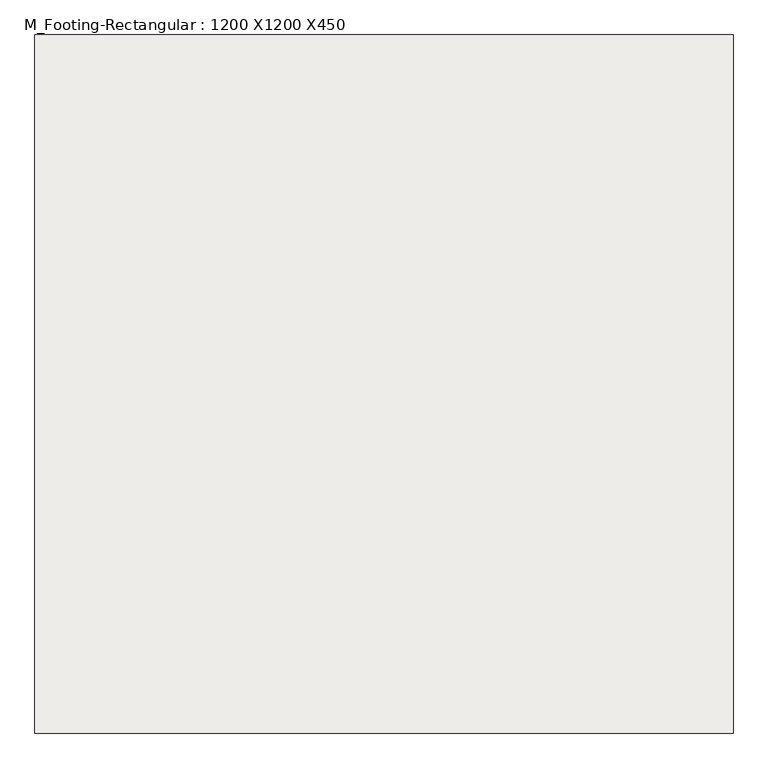
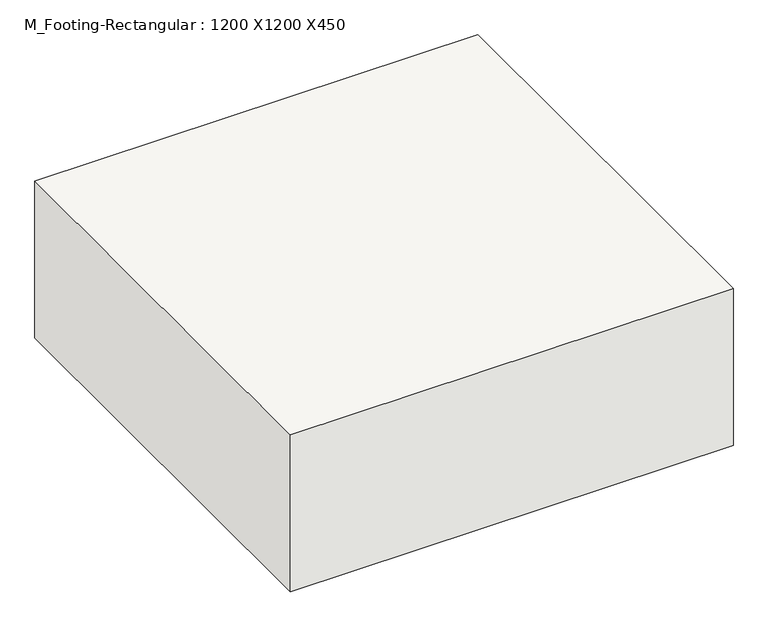
"""IFC4 building model written with IfcOpenShell, lengths in millimetres: slab geometry, M_Footing-Rectangular : 1200 X1200 X450."""

from ifc_helpers import new_model, si_unit, frame, origin, place, context, project, spatial, polyline, outline, extrude, source, transform, mapped, element, save


def m_footing_rectangular_1200_x1200_x450_1789818b(model_context):
    return source(origin(), model_context, "Body", "SweptSolid", [
        extrude(outline(polyline([(600.0, 600.0), (600.0, -600.0), (-600.0, -600.0), (-600.0, 600.0), (600.0, 600.0)])), frame((0.0, 0.0, -450.0), z_axis=(0.0, 0.0, 1.0), x_axis=(1.0, 0.0, 0.0)), (0.0, 0.0, 1.0), 450.0),
    ])


if __name__ == "__main__":
    model = new_model("IFC4")
    model_context = context("Model", 3, world=origin())
    ifc_project = project(units=[si_unit("LENGTHUNIT", "METRE", prefix="MILLI")], contexts=[model_context])
    site = spatial("IfcSite", under=ifc_project)
    building = spatial("IfcBuilding", under=site)
    placement = place(None, origin())
    m_footing_rectangular_1200_x1200_x450_shape = m_footing_rectangular_1200_x1200_x450_1789818b(model_context)
    element("IfcSlab", 1, ObjectType="M_Footing-Rectangular : 1200 X1200 X450", at=placement, inside=building, context=model_context, shape_type="MappedRepresentation", body=[
        mapped(m_footing_rectangular_1200_x1200_x450_shape, transform((0.0, 0.0, 0.0), x_axis=(1.0, 0.0, 0.0), y_axis=(0.0, 1.0, 0.0), z_axis=(0.0, 0.0, 1.0))),
    ])
    save(model, "model.ifc")

# Revit data of these elements
# Type "M_Footing-Rectangular : 1200 X1200 X450"
#   Width = 3' - 11.24409"
#   Length = 3' - 11.24409"
#   Foundation Thickness = 1' - 5.71654"
#   Structural Material [instance default] = Concrete, Cast-in-Place gray
#   Assembly Code = ""
# Element 1 (IfcSlab, "M_Footing-Rectangular : 1200 X1200 X450")
#   Materials on its faces: "Concrete, Cast-in-Place gray"
# Materials
#   "Concrete, Cast-in-Place gray": class "Concrete", colour RGB 192 192 192, transparency 0, Description = "Cast-in-place concrete", Cost = 0
